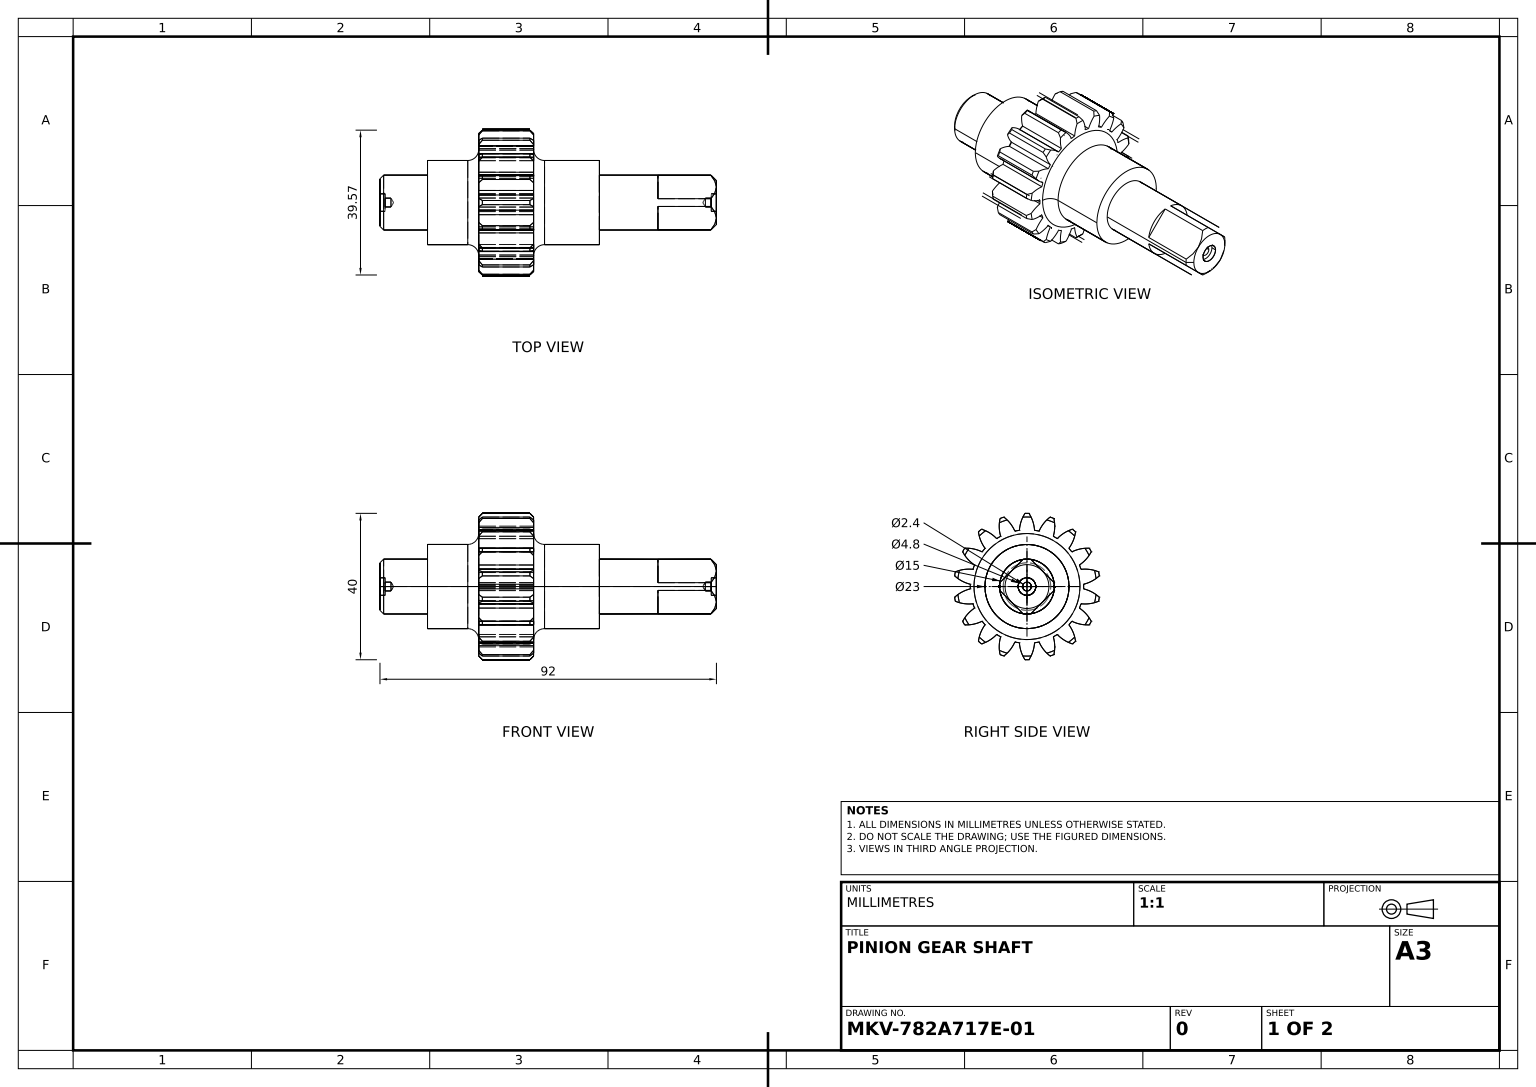
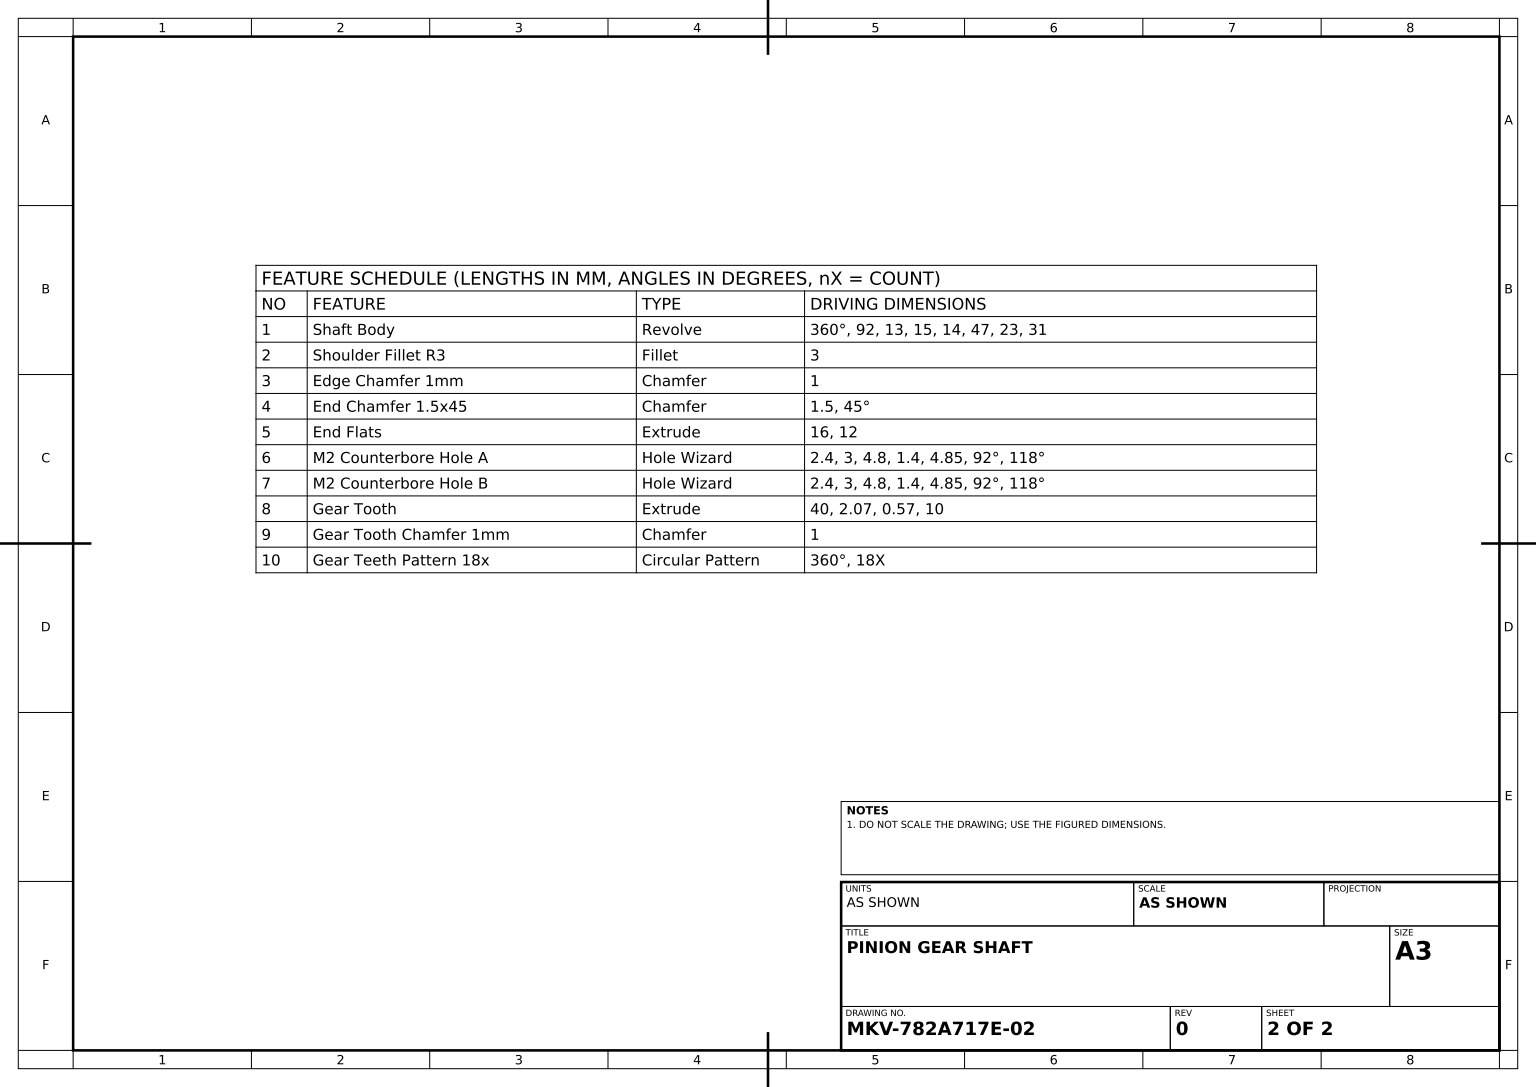
from build123d import *

# Parameters (mm, degrees)
SHOULDER_FILLET_R3_R                          = 3
EDGE_CHAMFER_1MM_SIZE                         = 1
END_CHAMFER_1_5X45_SIZE                       = 1.5
END_FLATS_DEPTH                               = 16
GEAR_TOOTH_DEPTH                              = 15
GEAR_TOOTH_CHAMFER_1MM_SIZE                   = 1
GEAR_TEETH_PATTERN_18X_COUNT                  = 18
GEAR_TOOTH_CHAMFER_1MM_OF_GEAR_TEETH_PAT_SIZE = 1


with BuildPart() as part:
    # Shaft Profile → Shaft Body (revolve)
    with BuildSketch(Plane.XY, mode=Mode.PRIVATE) as shaft_body_sk:
        Polygon((-34.5, 0), (-34.5, -7.5), (-21.5, -7.5), (-21.5, -11.5), (-7.5, -11.5), (-7.5, -15.5), (7.5, -15.5), (7.5, -11.5), (25.5, -11.5), (25.5, -7.5), (57.5, -7.5), (57.5, 0), align=None)
    revolve(shaft_body_sk.sketch.rotate(Axis((-34.5, 0, 0), (1, 0, 0)), 270), axis=Axis((-34.5, 0, 0), (1, 0, 0)))

    # Shoulder Fillet R3
    shoulder_fillet_r3_edges = [part.edges().sort_by_distance(p)[0] for p in [
        (7.5, 0, -11.5),
        (-7.5, 0, -11.5),
    ]]
    fillet(shoulder_fillet_r3_edges, radius=SHOULDER_FILLET_R3_R)

    # Edge Chamfer 1mm
    edge_chamfer_1mm_edges = [part.edges().sort_by_distance(p)[0] for p in [
        (-34.5, 0, -7.5),
    ]]
    chamfer(edge_chamfer_1mm_edges, length=EDGE_CHAMFER_1MM_SIZE)

    # End Chamfer 1.5x45
    end_chamfer_1_5x45_edges = [part.edges().sort_by_distance(p)[0] for p in [
        (57.5, 0, -7.5),
    ]]
    chamfer(end_chamfer_1_5x45_edges, length=END_CHAMFER_1_5X45_SIZE)

    # End Flats Profile → End Flats (cut)
    with BuildSketch(Plane(origin=(57.5, 0, 0), x_dir=(0, 0, -1), z_dir=(1, 0, 0))):
        with BuildLine():
            ThreePointArc((-1.060660172, 7.424621202), (-5.303300859, 5.303300859), (-7.424621202, 1.060660172))
            Line((-7.424621202, 1.060660172), (-1.060660172, 7.424621202))
        make_face()
        with BuildLine():
            ThreePointArc((-7.424621202, -1.060660172), (-5.303300859, -5.303300859), (-1.060660172, -7.424621202))
            Line((-1.060660172, -7.424621202), (-7.424621202, -1.060660172))
        make_face()
        with BuildLine():
            Line((7.424621202, -1.060660172), (1.060660172, -7.424621202))
            ThreePointArc((1.060660172, -7.424621202), (5.303300859, -5.303300859), (7.424621202, -1.060660172))
        make_face()
        with BuildLine():
            Line((1.060660172, 7.424621202), (7.424621202, 1.060660172))
            ThreePointArc((7.424621202, 1.060660172), (5.303300859, 5.303300859), (1.060660172, 7.424621202))
        make_face()
    extrude(amount=-END_FLATS_DEPTH, mode=Mode.SUBTRACT)

    # Sketch5 → M2 Counterbore Hole A (revolve, cut)
    with BuildSketch(Plane(origin=(57.5, 0, 0), x_dir=(0, 0, -1), z_dir=(0, 1, 0))):
        Polygon((0, 0), (0, 3.721032743), (1.2, 3), (1.2, 1.4), (2.4, 1.4), (2.4, 0.024142219), (2.425, 0), align=None)
    revolve(axis=Axis((63.85, 0, 0), (-1, 0, 0)), mode=Mode.SUBTRACT)

    # Sketch7 → M2 Counterbore Hole B (revolve, cut)
    with BuildSketch(Plane(origin=(-34.5, 0, 0), x_dir=(0, 0, 1), z_dir=(0, 1, 0))):
        Polygon((0, 0), (0, 3.721032743), (1.2, 3), (1.2, 1.4), (2.4, 1.4), (2.4, 0.024142219), (2.425, 0), align=None)
    revolve(axis=Axis((-40.85, 0, 0), (1, 0, 0)), mode=Mode.SUBTRACT)

    # Gear Tooth Profile → Gear Tooth (add)
    with BuildSketch(Plane(origin=(7.5, 0, 0), x_dir=(0, 0, -1), z_dir=(1, 0, 0))):
        with BuildLine():
            ThreePointArc((0.57, 19.99187585), (0, 20), (-0.57, 19.99187585))
            ThreePointArc((-0.57, 19.99187585), (-1.60605715, 17.76917639), (-2.07, 15.361155555))
            ThreePointArc((-2.07, 15.361155555), (0, 15.5), (2.07, 15.361155555))
            ThreePointArc((2.07, 15.361155555), (1.60605715, 17.76917639), (0.57, 19.99187585))
        make_face()
    gear_tooth = extrude(amount=-GEAR_TOOTH_DEPTH)

    # Gear Tooth Chamfer 1mm
    gear_tooth_chamfer_1mm_edges = [part.edges().sort_by_distance(p)[0] for p in [
        (7.5, 20, 0),
        (-7.5, 20, 0),
    ]]
    chamfer(gear_tooth_chamfer_1mm_edges, length=GEAR_TOOTH_CHAMFER_1MM_SIZE)

    # Gear Teeth Pattern 18x: Gear Tooth ×18 about axis
    gear_teeth_pattern_18x_axis = Axis((0, 0, 0), (1, 0, 0))
    for i in range(1, GEAR_TEETH_PATTERN_18X_COUNT):
        add(gear_tooth.rotate(gear_teeth_pattern_18x_axis, i * 360 / GEAR_TEETH_PATTERN_18X_COUNT))

    # Gear Tooth Chamfer 1mm of Gear Teeth Pat
    gear_tooth_chamfer_1mm_of_gear_teeth_pat_edges = [part.edges().sort_by_distance(p)[0] for p in [
        (7.5, 18.793852416, 6.840402867),
        (-7.5, 18.793852416, 6.840402867),
        (7.5, 15.320888862, 12.855752194),
        (-7.5, 15.320888862, 12.855752194),
        (7.5, 10, 17.320508076),
        (-7.5, 10, 17.320508076),
        (7.5, 3.472963553, 19.69615506),
        (-7.5, 3.472963553, 19.69615506),
        (7.5, -3.472963553, 19.69615506),
        (-7.5, -3.472963553, 19.69615506),
        (7.5, -10, 17.320508076),
        (-7.5, -10, 17.320508076),
        (7.5, -15.320888862, 12.855752194),
        (-7.5, -15.320888862, 12.855752194),
        (7.5, -18.793852416, 6.840402867),
        (-7.5, -18.793852416, 6.840402867),
        (7.5, -20, 0),
        (-7.5, -20, 0),
        (7.5, -18.793852416, -6.840402867),
        (-7.5, -18.793852416, -6.840402867),
        (7.5, -15.320888862, -12.855752194),
        (-7.5, -15.320888862, -12.855752194),
        (7.5, -10, -17.320508076),
        (-7.5, -10, -17.320508076),
        (7.5, -3.472963553, -19.69615506),
        (-7.5, -3.472963553, -19.69615506),
        (7.5, 3.472963553, -19.69615506),
        (-7.5, 3.472963553, -19.69615506),
        (7.5, 10, -17.320508076),
        (-7.5, 10, -17.320508076),
        (7.5, 15.320888862, -12.855752194),
        (-7.5, 15.320888862, -12.855752194),
        (7.5, 18.793852416, -6.840402867),
        (-7.5, 18.793852416, -6.840402867),
    ]]
    chamfer(gear_tooth_chamfer_1mm_of_gear_teeth_pat_edges, length=GEAR_TOOTH_CHAMFER_1MM_OF_GEAR_TEETH_PAT_SIZE)


solid = part.part
